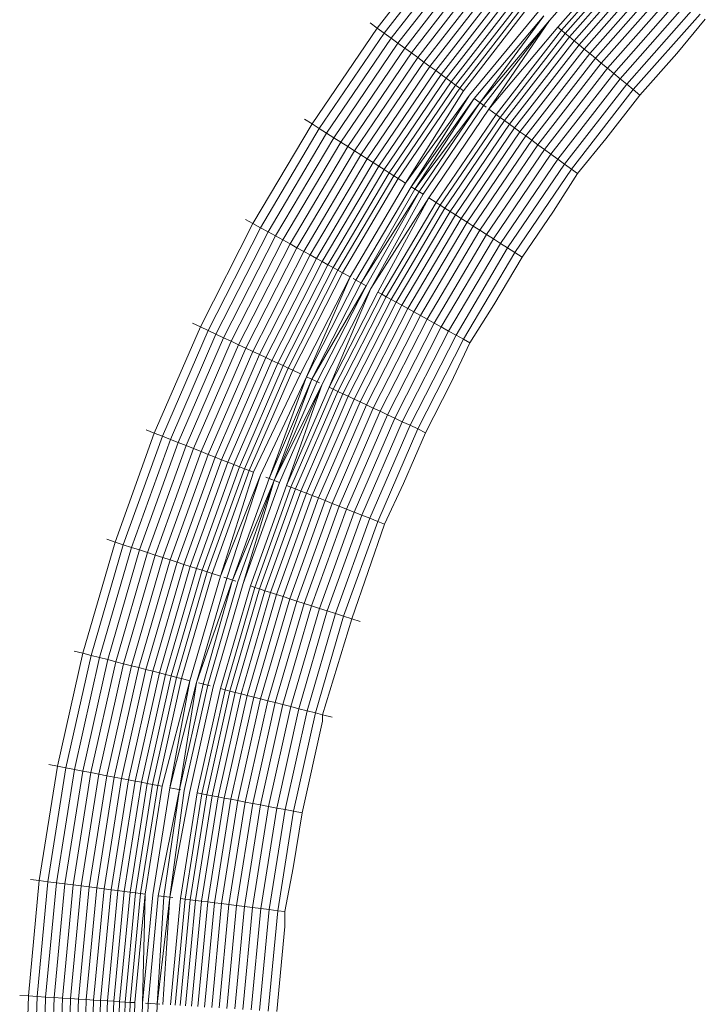
# Model space of a CAD drawing. Units: inches. Extents: x 64 to 1167, y 117 to 939.
# Tile 45 of 56: x 1129.7649 to 1129.9466, y 500.9712 to 501.2323. Entities that reach past the tile are written whole.
import ezdxf

# ---------------------------------------------------------------- set-up
doc = ezdxf.new("R2010")
doc.units = ezdxf.units.IN
doc.header["$MEASUREMENT"] = 0
doc.layers.add('A-FLOR-FIXT', color=8, linetype='Continuous', lineweight=18)

msp = doc.modelspace()

# ---------------------------------------------------------------- linework, layer by layer
at = {"layer": 'A-FLOR-FIXT'}
for p, q in [((1129.87845, 501.25434), (1129.85963, 501.23007)), ((1129.88022, 501.25287), (1129.86149, 501.22872)), ((1129.88198, 501.25142), (1129.86333, 501.22738)), ((1129.92417, 501.25352), (1129.90531, 501.23212)), ((1129.92626, 501.25156), (1129.90751, 501.2303)), ((1129.88371, 501.24999), (1129.86515, 501.22606)), ((1129.88542, 501.24858), (1129.86694, 501.22476)), ((1129.92714, 501.25073), (1129.90845, 501.22952)), ((1129.92812, 501.24981), (1129.90949, 501.22867)), ((1129.92919, 501.2488), (1129.91062, 501.22773)), ((1129.88708, 501.2472), (1129.86869, 501.22349)), ((1129.8887, 501.24586), (1129.87039, 501.22225)), ((1129.93034, 501.24772), (1129.91183, 501.22673)), ((1129.93157, 501.24657), (1129.91313, 501.22565)), ((1129.89027, 501.24456), (1129.87204, 501.22106)), ((1129.89178, 501.24331), (1129.87362, 501.2199)), ((1129.93287, 501.24535), (1129.91451, 501.22451)), ((1129.93424, 501.24406), (1129.91595, 501.22332)), ((1129.89323, 501.24212), (1129.87514, 501.2188)), ((1129.8946, 501.24098), (1129.87659, 501.21775)), ((1129.93567, 501.24272), (1129.91746, 501.22207)), ((1129.93716, 501.24132), (1129.91903, 501.22077)), ((1129.8959, 501.2399), (1129.87795, 501.21676)), ((1129.89712, 501.2389), (1129.87923, 501.21583)), ((1129.93869, 501.23988), (1129.92065, 501.21943)), ((1129.94027, 501.2384), (1129.92232, 501.21805)), ((1129.89825, 501.23796), (1129.88041, 501.21497)), ((1129.89928, 501.23711), (1129.8815, 501.21418)), ((1129.90022, 501.23633), (1129.88249, 501.21346)), ((1129.94188, 501.23689), (1129.92402, 501.21664)), ((1129.90242, 501.23451), (1129.88414, 501.21226)), ((1129.90381, 501.23336), (1129.88534, 501.21139)), ((1129.90381, 501.23336), (1129.88686, 501.21029)), ((1129.94352, 501.23535), (1129.92576, 501.21521)), ((1129.94518, 501.23379), (1129.92751, 501.21375)), ((1129.85963, 501.23007), (1129.85776, 501.23143)), ((1129.90531, 501.23212), (1129.88686, 501.21029)), ((1129.90531, 501.23212), (1129.88783, 501.20958)), ((1129.90531, 501.23212), (1129.88926, 501.20854)), ((1129.90751, 501.2303), (1129.88926, 501.20854)), ((1129.90845, 501.22952), (1129.90751, 501.2303)), ((1129.94658, 501.23247), (1129.93901, 501.22333)), ((1129.85963, 501.23007), (1129.84237, 501.20467)), ((1129.86149, 501.22872), (1129.84431, 501.20344)), ((1129.86149, 501.22872), (1129.85963, 501.23007)), ((1129.86333, 501.22738), (1129.86149, 501.22872)), ((1129.90845, 501.22952), (1129.89113, 501.20719)), ((1129.90949, 501.22867), (1129.89221, 501.2064)), ((1129.91062, 501.22773), (1129.8934, 501.20554)), ((1129.90949, 501.22867), (1129.90845, 501.22952)), ((1129.91062, 501.22773), (1129.90949, 501.22867)), ((1129.91183, 501.22673), (1129.91062, 501.22773)), ((1129.86333, 501.22738), (1129.84623, 501.20222)), ((1129.86515, 501.22606), (1129.84813, 501.20101)), ((1129.86515, 501.22606), (1129.86333, 501.22738)), ((1129.86694, 501.22476), (1129.86515, 501.22606)), ((1129.91183, 501.22673), (1129.89468, 501.20461)), ((1129.91313, 501.22565), (1129.89604, 501.20362)), ((1129.91313, 501.22565), (1129.91183, 501.22673)), ((1129.91451, 501.22451), (1129.91313, 501.22565)), ((1129.86694, 501.22476), (1129.85, 501.19983)), ((1129.86869, 501.22349), (1129.85182, 501.19867)), ((1129.86869, 501.22349), (1129.86694, 501.22476)), ((1129.87039, 501.22225), (1129.86869, 501.22349)), ((1129.91451, 501.22451), (1129.89748, 501.20257)), ((1129.91595, 501.22332), (1129.899, 501.20146)), ((1129.91595, 501.22332), (1129.91451, 501.22451)), ((1129.91746, 501.22207), (1129.91595, 501.22332)), ((1129.93901, 501.22333), (1129.92928, 501.21229)), ((1129.87039, 501.22225), (1129.8536, 501.19754)), ((1129.87204, 501.22106), (1129.85532, 501.19645)), ((1129.87362, 501.2199), (1129.85697, 501.1954)), ((1129.87204, 501.22106), (1129.87039, 501.22225)), ((1129.87362, 501.2199), (1129.87204, 501.22106)), ((1129.87514, 501.2188), (1129.87362, 501.2199)), ((1129.91746, 501.22207), (1129.90059, 501.20031)), ((1129.91903, 501.22077), (1129.90224, 501.19911)), ((1129.91903, 501.22077), (1129.91746, 501.22207)), ((1129.92065, 501.21943), (1129.91903, 501.22077)), ((1129.87514, 501.2188), (1129.85856, 501.19439)), ((1129.87659, 501.21775), (1129.86006, 501.19344)), ((1129.87659, 501.21775), (1129.87514, 501.2188)), ((1129.87795, 501.21676), (1129.87659, 501.21775)), ((1129.92065, 501.21943), (1129.90394, 501.19788)), ((1129.92232, 501.21805), (1129.90569, 501.19661)), ((1129.92232, 501.21805), (1129.92065, 501.21943)), ((1129.92402, 501.21664), (1129.92232, 501.21805)), ((1129.87795, 501.21676), (1129.86149, 501.19253)), ((1129.87923, 501.21583), (1129.86282, 501.19169)), ((1129.88041, 501.21497), (1129.86406, 501.1909)), ((1129.87923, 501.21583), (1129.87795, 501.21676)), ((1129.88041, 501.21497), (1129.87923, 501.21583)), ((1129.8815, 501.21418), (1129.88041, 501.21497)), ((1129.92402, 501.21664), (1129.90748, 501.19531)), ((1129.92576, 501.21521), (1129.9093, 501.19399)), ((1129.92576, 501.21521), (1129.92402, 501.21664)), ((1129.92751, 501.21375), (1129.92576, 501.21521)), ((1129.8815, 501.21418), (1129.86519, 501.19018)), ((1129.88249, 501.21346), (1129.86714, 501.18895)), ((1129.88414, 501.21226), (1129.86714, 501.18895)), ((1129.88414, 501.21226), (1129.86863, 501.188)), ((1129.88249, 501.21346), (1129.8815, 501.21418)), ((1129.92751, 501.21375), (1129.91114, 501.19265)), ((1129.92928, 501.21229), (1129.92026, 501.20066)), ((1129.92928, 501.21229), (1129.92751, 501.21375)), ((1129.88534, 501.21139), (1129.86863, 501.188)), ((1129.88534, 501.21139), (1129.86964, 501.18736)), ((1129.88686, 501.21029), (1129.86964, 501.18736)), ((1129.88686, 501.21029), (1129.87079, 501.18663)), ((1129.88783, 501.20958), (1129.8718, 501.18599)), ((1129.88534, 501.21139), (1129.88849, 501.2091)), ((1129.88926, 501.20854), (1129.87329, 501.18505)), ((1129.89113, 501.20719), (1129.87524, 501.18381)), ((1129.88926, 501.20854), (1129.89113, 501.20719)), ((1129.89113, 501.20719), (1129.89221, 501.2064)), ((1129.84237, 501.20467), (1129.82673, 501.17823)), ((1129.84237, 501.20467), (1129.84042, 501.20591)), ((1129.84431, 501.20344), (1129.84237, 501.20467)), ((1129.89221, 501.2064), (1129.87637, 501.18309)), ((1129.8934, 501.20554), (1129.87761, 501.1823)), ((1129.89468, 501.20461), (1129.87894, 501.18146)), ((1129.8934, 501.20554), (1129.89221, 501.2064)), ((1129.89468, 501.20461), (1129.8934, 501.20554)), ((1129.89604, 501.20362), (1129.89468, 501.20461)), ((1129.84431, 501.20344), (1129.82875, 501.17713)), ((1129.84623, 501.20222), (1129.83074, 501.17603)), ((1129.84623, 501.20222), (1129.84431, 501.20344)), ((1129.84813, 501.20101), (1129.84623, 501.20222)), ((1129.89604, 501.20362), (1129.88037, 501.18055)), ((1129.89748, 501.20257), (1129.88187, 501.1796)), ((1129.899, 501.20146), (1129.88346, 501.17859)), ((1129.89748, 501.20257), (1129.89604, 501.20362)), ((1129.899, 501.20146), (1129.89748, 501.20257)), ((1129.90059, 501.20031), (1129.899, 501.20146)), ((1129.84813, 501.20101), (1129.83271, 501.17494)), ((1129.85, 501.19983), (1129.83465, 501.17388)), ((1129.85, 501.19983), (1129.84813, 501.20101)), ((1129.85182, 501.19867), (1129.85, 501.19983)), ((1129.90059, 501.20031), (1129.88511, 501.17754)), ((1129.90224, 501.19911), (1129.88683, 501.17645)), ((1129.90224, 501.19911), (1129.90059, 501.20031)), ((1129.90394, 501.19788), (1129.90224, 501.19911)), ((1129.92026, 501.20066), (1129.9127, 501.19152)), ((1129.85182, 501.19867), (1129.83654, 501.17284)), ((1129.8536, 501.19754), (1129.83839, 501.17183)), ((1129.85532, 501.19645), (1129.84017, 501.17084)), ((1129.8536, 501.19754), (1129.85182, 501.19867)), ((1129.85532, 501.19645), (1129.8536, 501.19754)), ((1129.85697, 501.1954), (1129.85532, 501.19645)), ((1129.90394, 501.19788), (1129.88861, 501.17532)), ((1129.90569, 501.19661), (1129.89043, 501.17416)), ((1129.90569, 501.19661), (1129.90394, 501.19788)), ((1129.90748, 501.19531), (1129.90569, 501.19661)), ((1129.85697, 501.1954), (1129.84189, 501.1699)), ((1129.85856, 501.19439), (1129.84354, 501.16899)), ((1129.85856, 501.19439), (1129.85697, 501.1954)), ((1129.86006, 501.19344), (1129.85856, 501.19439)), ((1129.90748, 501.19531), (1129.8923, 501.17298)), ((1129.9093, 501.19399), (1129.8942, 501.17177)), ((1129.9093, 501.19399), (1129.90748, 501.19531)), ((1129.91114, 501.19265), (1129.9093, 501.19399)), ((1129.86006, 501.19344), (1129.8451, 501.16813)), ((1129.86149, 501.19253), (1129.84658, 501.16732)), ((1129.86282, 501.19169), (1129.84796, 501.16656)), ((1129.86149, 501.19253), (1129.86006, 501.19344)), ((1129.86282, 501.19169), (1129.86149, 501.19253)), ((1129.86406, 501.1909), (1129.86282, 501.19169)), ((1129.91114, 501.19265), (1129.89612, 501.17055)), ((1129.9127, 501.19152), (1129.90634, 501.18149)), ((1129.9127, 501.19152), (1129.91114, 501.19265)), ((1129.86406, 501.1909), (1129.84924, 501.16586)), ((1129.86519, 501.19018), (1129.85042, 501.16521)), ((1129.86714, 501.18895), (1129.85245, 501.1641)), ((1129.86519, 501.19018), (1129.86406, 501.1909)), ((1129.86714, 501.18895), (1129.86519, 501.19018)), ((1129.86863, 501.188), (1129.85399, 501.16325)), ((1129.86964, 501.18736), (1129.85537, 501.16249)), ((1129.87079, 501.18663), (1129.85537, 501.16249)), ((1129.87079, 501.18663), (1129.85669, 501.16176)), ((1129.8718, 501.18599), (1129.85799, 501.16105)), ((1129.86863, 501.188), (1129.8718, 501.18599)), ((1129.87329, 501.18505), (1129.85799, 501.16105)), ((1129.87329, 501.18505), (1129.85978, 501.16007)), ((1129.87524, 501.18381), (1129.86085, 501.15948)), ((1129.87524, 501.18381), (1129.87329, 501.18505)), ((1129.87637, 501.18309), (1129.87524, 501.18381)), ((1129.87637, 501.18309), (1129.86203, 501.15883)), ((1129.87761, 501.1823), (1129.86331, 501.15812)), ((1129.87894, 501.18146), (1129.86469, 501.15736)), ((1129.87761, 501.1823), (1129.87637, 501.18309)), ((1129.87894, 501.18146), (1129.87761, 501.1823)), ((1129.88037, 501.18055), (1129.87894, 501.18146)), ((1129.90634, 501.18149), (1129.89806, 501.16932)), ((1129.82673, 501.17823), (1129.81279, 501.15087)), ((1129.82673, 501.17823), (1129.82471, 501.17935)), ((1129.82875, 501.17713), (1129.82673, 501.17823)), ((1129.88037, 501.18055), (1129.86617, 501.15655)), ((1129.88187, 501.1796), (1129.86774, 501.15569)), ((1129.88346, 501.17859), (1129.86938, 501.15479)), ((1129.88187, 501.1796), (1129.88037, 501.18055)), ((1129.88346, 501.17859), (1129.88187, 501.1796)), ((1129.88511, 501.17754), (1129.88346, 501.17859)), ((1129.82875, 501.17713), (1129.81487, 501.14989)), ((1129.83074, 501.17603), (1129.81693, 501.14892)), ((1129.83074, 501.17603), (1129.82875, 501.17713)), ((1129.83271, 501.17494), (1129.83074, 501.17603)), ((1129.88511, 501.17754), (1129.8711, 501.15384)), ((1129.88683, 501.17645), (1129.87288, 501.15286)), ((1129.88683, 501.17645), (1129.88511, 501.17754)), ((1129.88861, 501.17532), (1129.88683, 501.17645)), ((1129.83271, 501.17494), (1129.81896, 501.14796)), ((1129.83465, 501.17388), (1129.82096, 501.14702)), ((1129.83654, 501.17284), (1129.82292, 501.1461)), ((1129.83465, 501.17388), (1129.83271, 501.17494)), ((1129.83654, 501.17284), (1129.83465, 501.17388)), ((1129.83839, 501.17183), (1129.83654, 501.17284)), ((1129.88861, 501.17532), (1129.87473, 501.15185)), ((1129.89043, 501.17416), (1129.87662, 501.15081)), ((1129.8923, 501.17298), (1129.87856, 501.14974)), ((1129.89043, 501.17416), (1129.88861, 501.17532)), ((1129.8923, 501.17298), (1129.89043, 501.17416)), ((1129.8942, 501.17177), (1129.8923, 501.17298)), ((1129.83839, 501.17183), (1129.82482, 501.1452)), ((1129.84017, 501.17084), (1129.82667, 501.14434)), ((1129.84017, 501.17084), (1129.83839, 501.17183)), ((1129.84189, 501.1699), (1129.84017, 501.17084)), ((1129.8942, 501.17177), (1129.88053, 501.14866)), ((1129.89612, 501.17055), (1129.88253, 501.14756)), ((1129.89612, 501.17055), (1129.8942, 501.17177)), ((1129.89806, 501.16932), (1129.89612, 501.17055)), ((1129.84189, 501.1699), (1129.82844, 501.1435)), ((1129.84354, 501.16899), (1129.83014, 501.1427)), ((1129.8451, 501.16813), (1129.83175, 501.14194)), ((1129.84354, 501.16899), (1129.84189, 501.1699)), ((1129.8451, 501.16813), (1129.84354, 501.16899)), ((1129.84658, 501.16732), (1129.8451, 501.16813)), ((1129.89806, 501.16932), (1129.89057, 501.15666)), ((1129.84658, 501.16732), (1129.83328, 501.14123)), ((1129.84796, 501.16656), (1129.83471, 501.14055)), ((1129.84924, 501.16586), (1129.83603, 501.13993)), ((1129.85042, 501.16521), (1129.83725, 501.13936)), ((1129.84796, 501.16656), (1129.84658, 501.16732)), ((1129.84924, 501.16586), (1129.84796, 501.16656)), ((1129.85042, 501.16521), (1129.84924, 501.16586)), ((1129.85245, 501.1641), (1129.85042, 501.16521)), ((1129.85245, 501.1641), (1129.83934, 501.13837)), ((1129.85245, 501.1641), (1129.84094, 501.13762)), ((1129.85399, 501.16325), (1129.84094, 501.13762)), ((1129.85537, 501.16249), (1129.84236, 501.13695)), ((1129.85328, 501.16364), (1129.85669, 501.16176)), ((1129.85669, 501.16176), (1129.84236, 501.13695)), ((1129.85669, 501.16176), (1129.84372, 501.13631)), ((1129.85799, 501.16105), (1129.84506, 501.13568)), ((1129.85799, 501.16105), (1129.84691, 501.13481)), ((1129.85978, 501.16007), (1129.84691, 501.13481)), ((1129.86085, 501.15948), (1129.85978, 501.16007)), ((1129.86085, 501.15948), (1129.84801, 501.13429)), ((1129.86203, 501.15883), (1129.84923, 501.13372)), ((1129.86331, 501.15812), (1129.85056, 501.13309)), ((1129.86469, 501.15736), (1129.85199, 501.13242)), ((1129.86203, 501.15883), (1129.86085, 501.15948)), ((1129.86331, 501.15812), (1129.86203, 501.15883)), ((1129.86469, 501.15736), (1129.86331, 501.15812)), ((1129.86617, 501.15655), (1129.86469, 501.15736)), ((1129.86617, 501.15655), (1129.85351, 501.1317)), ((1129.86774, 501.15569), (1129.85513, 501.13094)), ((1129.86938, 501.15479), (1129.85683, 501.13015)), ((1129.86774, 501.15569), (1129.86617, 501.15655)), ((1129.86938, 501.15479), (1129.86774, 501.15569)), ((1129.8711, 501.15384), (1129.86938, 501.15479)), ((1129.89057, 501.15666), (1129.88421, 501.14663)), ((1129.81279, 501.15087), (1129.8107, 501.15185)), ((1129.8711, 501.15384), (1129.8586, 501.12931)), ((1129.87288, 501.15286), (1129.86044, 501.12844)), ((1129.87473, 501.15185), (1129.86235, 501.12755)), ((1129.87288, 501.15286), (1129.8711, 501.15384)), ((1129.87473, 501.15185), (1129.87288, 501.15286)), ((1129.87662, 501.15081), (1129.87473, 501.15185)), ((1129.81279, 501.15087), (1129.80059, 501.12268)), ((1129.81487, 501.14989), (1129.80273, 501.12183)), ((1129.81487, 501.14989), (1129.81279, 501.15087)), ((1129.81693, 501.14892), (1129.81487, 501.14989)), ((1129.87662, 501.15081), (1129.8643, 501.12663)), ((1129.87856, 501.14974), (1129.8663, 501.12569)), ((1129.87856, 501.14974), (1129.87662, 501.15081)), ((1129.88053, 501.14866), (1129.87856, 501.14974)), ((1129.81693, 501.14892), (1129.80485, 501.121)), ((1129.81896, 501.14796), (1129.80694, 501.12017)), ((1129.82096, 501.14702), (1129.80899, 501.11935)), ((1129.81896, 501.14796), (1129.81693, 501.14892)), ((1129.82096, 501.14702), (1129.81896, 501.14796)), ((1129.82292, 501.1461), (1129.82096, 501.14702)), ((1129.88053, 501.14866), (1129.86834, 501.12473)), ((1129.88253, 501.14756), (1129.8704, 501.12376)), ((1129.88421, 501.14663), (1129.87916, 501.13589)), ((1129.88253, 501.14756), (1129.88053, 501.14866)), ((1129.88421, 501.14663), (1129.88253, 501.14756)), ((1129.82292, 501.1461), (1129.811, 501.11856)), ((1129.82482, 501.1452), (1129.81296, 501.11778)), ((1129.82667, 501.14434), (1129.81485, 501.11703)), ((1129.82482, 501.1452), (1129.82292, 501.1461)), ((1129.82667, 501.14434), (1129.82482, 501.1452)), ((1129.82844, 501.1435), (1129.82667, 501.14434)), ((1129.82844, 501.1435), (1129.81667, 501.11631)), ((1129.83014, 501.1427), (1129.81842, 501.11562)), ((1129.83175, 501.14194), (1129.82008, 501.11496)), ((1129.83014, 501.1427), (1129.82844, 501.1435)), ((1129.83175, 501.14194), (1129.83014, 501.1427)), ((1129.83328, 501.14123), (1129.83175, 501.14194)), ((1129.83328, 501.14123), (1129.82165, 501.11434)), ((1129.83471, 501.14055), (1129.82312, 501.11376)), ((1129.83603, 501.13993), (1129.82448, 501.11322)), ((1129.83725, 501.13936), (1129.82573, 501.11273)), ((1129.83471, 501.14055), (1129.83328, 501.14123)), ((1129.83603, 501.13993), (1129.83471, 501.14055)), ((1129.83725, 501.13936), (1129.83603, 501.13993)), ((1129.83934, 501.13837), (1129.83725, 501.13936)), ((1129.83934, 501.13837), (1129.82686, 501.11228)), ((1129.84094, 501.13762), (1129.82876, 501.11153)), ((1129.84094, 501.13762), (1129.83098, 501.11065)), ((1129.84236, 501.13695), (1129.83098, 501.11065)), ((1129.84236, 501.13695), (1129.83238, 501.1101)), ((1129.84372, 501.13631), (1129.83238, 501.1101)), ((1129.84094, 501.13762), (1129.84433, 501.13603)), ((1129.84506, 501.13568), (1129.83238, 501.1101)), ((1129.84506, 501.13568), (1129.83376, 501.10955)), ((1129.84506, 501.13568), (1129.83565, 501.1088)), ((1129.84691, 501.13481), (1129.83565, 501.1088)), ((1129.84801, 501.13429), (1129.83679, 501.10835)), ((1129.84923, 501.13372), (1129.83804, 501.10785)), ((1129.84691, 501.13481), (1129.84801, 501.13429)), ((1129.84801, 501.13429), (1129.84923, 501.13372)), ((1129.84923, 501.13372), (1129.85056, 501.13309)), ((1129.87916, 501.13589), (1129.87248, 501.12278)), ((1129.85056, 501.13309), (1129.8394, 501.10731)), ((1129.85199, 501.13242), (1129.84087, 501.10673)), ((1129.85351, 501.1317), (1129.84244, 501.10611)), ((1129.85056, 501.13309), (1129.85199, 501.13242)), ((1129.85351, 501.1317), (1129.85199, 501.13242)), ((1129.85513, 501.13094), (1129.85351, 501.1317)), ((1129.85513, 501.13094), (1129.8441, 501.10546)), ((1129.85683, 501.13015), (1129.84584, 501.10476)), ((1129.8586, 501.12931), (1129.84767, 501.10404)), ((1129.86044, 501.12844), (1129.84956, 501.10329)), ((1129.85683, 501.13015), (1129.85513, 501.13094)), ((1129.8586, 501.12931), (1129.85683, 501.13015)), ((1129.86044, 501.12844), (1129.8586, 501.12931)), ((1129.86235, 501.12755), (1129.86044, 501.12844)), ((1129.86235, 501.12755), (1129.85151, 501.10252)), ((1129.8643, 501.12663), (1129.85352, 501.10172)), ((1129.8643, 501.12663), (1129.86235, 501.12755)), ((1129.8663, 501.12569), (1129.8643, 501.12663)), ((1129.80059, 501.12268), (1129.79844, 501.12353)), ((1129.8663, 501.12569), (1129.85558, 501.10091)), ((1129.86834, 501.12473), (1129.85767, 501.10008)), ((1129.8704, 501.12376), (1129.85979, 501.09924)), ((1129.86834, 501.12473), (1129.8663, 501.12569)), ((1129.8704, 501.12376), (1129.86834, 501.12473)), ((1129.87248, 501.12278), (1129.8704, 501.12376)), ((1129.80059, 501.12268), (1129.79019, 501.09378)), ((1129.80273, 501.12183), (1129.79237, 501.09307)), ((1129.80485, 501.121), (1129.79454, 501.09237)), ((1129.80273, 501.12183), (1129.80059, 501.12268)), ((1129.80485, 501.121), (1129.80273, 501.12183)), ((1129.80694, 501.12017), (1129.80485, 501.121)), ((1129.87248, 501.12278), (1129.86663, 501.10928)), ((1129.80694, 501.12017), (1129.79668, 501.09167)), ((1129.80899, 501.11935), (1129.79878, 501.09099)), ((1129.811, 501.11856), (1129.80084, 501.09032)), ((1129.80899, 501.11935), (1129.80694, 501.12017)), ((1129.811, 501.11856), (1129.80899, 501.11935)), ((1129.81296, 501.11778), (1129.811, 501.11856)), ((1129.81296, 501.11778), (1129.80284, 501.08967)), ((1129.81485, 501.11703), (1129.80477, 501.08904)), ((1129.81667, 501.11631), (1129.80664, 501.08844)), ((1129.81842, 501.11562), (1129.80842, 501.08786)), ((1129.81485, 501.11703), (1129.81296, 501.11778)), ((1129.81667, 501.11631), (1129.81485, 501.11703)), ((1129.81842, 501.11562), (1129.81667, 501.11631)), ((1129.82008, 501.11496), (1129.81842, 501.11562)), ((1129.82008, 501.11496), (1129.81012, 501.08731)), ((1129.82165, 501.11434), (1129.81173, 501.08679)), ((1129.82312, 501.11376), (1129.81323, 501.0863)), ((1129.82448, 501.11322), (1129.81462, 501.08584)), ((1129.82573, 501.11273), (1129.8159, 501.08543)), ((1129.82165, 501.11434), (1129.82008, 501.11496)), ((1129.82312, 501.11376), (1129.82165, 501.11434)), ((1129.82448, 501.11322), (1129.82312, 501.11376)), ((1129.82573, 501.11273), (1129.82448, 501.11322)), ((1129.82686, 501.11228), (1129.82573, 501.11273)), ((1129.82686, 501.11228), (1129.8181, 501.08472)), ((1129.82876, 501.11153), (1129.8181, 501.08472)), ((1129.82876, 501.11153), (1129.81978, 501.08417)), ((1129.83098, 501.11065), (1129.82127, 501.08368)), ((1129.83238, 501.1101), (1129.82127, 501.08368)), ((1129.83238, 501.1101), (1129.8227, 501.08322)), ((1129.83238, 501.1101), (1129.82411, 501.08276)), ((1129.83014, 501.11098), (1129.83376, 501.10955)), ((1129.83376, 501.10955), (1129.82411, 501.08276)), ((1129.83565, 501.1088), (1129.82605, 501.08213)), ((1129.83679, 501.10835), (1129.82721, 501.08175)), ((1129.83804, 501.10785), (1129.82849, 501.08134)), ((1129.83679, 501.10835), (1129.83565, 501.1088)), ((1129.83804, 501.10785), (1129.83679, 501.10835)), ((1129.8394, 501.10731), (1129.83804, 501.10785)), ((1129.86663, 501.10928), (1129.86158, 501.09853)), ((1129.8394, 501.10731), (1129.82989, 501.08088)), ((1129.84087, 501.10673), (1129.83139, 501.0804)), ((1129.84244, 501.10611), (1129.83299, 501.07988)), ((1129.8441, 501.10546), (1129.83469, 501.07932)), ((1129.84087, 501.10673), (1129.8394, 501.10731)), ((1129.84244, 501.10611), (1129.84087, 501.10673)), ((1129.84244, 501.10611), (1129.8441, 501.10546)), ((1129.8441, 501.10546), (1129.84584, 501.10476)), ((1129.84584, 501.10476), (1129.83647, 501.07874)), ((1129.84767, 501.10404), (1129.83834, 501.07814)), ((1129.84956, 501.10329), (1129.84028, 501.07751)), ((1129.85151, 501.10252), (1129.84228, 501.07686)), ((1129.84584, 501.10476), (1129.84767, 501.10404)), ((1129.84767, 501.10404), (1129.84956, 501.10329)), ((1129.84956, 501.10329), (1129.85151, 501.10252)), ((1129.85151, 501.10252), (1129.85352, 501.10172)), ((1129.85352, 501.10172), (1129.84433, 501.07619)), ((1129.85558, 501.10091), (1129.84643, 501.07551)), ((1129.85767, 501.10008), (1129.84857, 501.07481)), ((1129.85352, 501.10172), (1129.85558, 501.10091)), ((1129.85558, 501.10091), (1129.85767, 501.10008)), ((1129.85767, 501.10008), (1129.85979, 501.09924)), ((1129.85979, 501.09924), (1129.85074, 501.07411)), ((1129.86158, 501.09853), (1129.85293, 501.0734)), ((1129.85979, 501.09924), (1129.86158, 501.09853)), ((1129.79019, 501.09378), (1129.78799, 501.0945)), ((1129.79019, 501.09378), (1129.78162, 501.06429)), ((1129.79237, 501.09307), (1129.78384, 501.06372)), ((1129.79454, 501.09237), (1129.78605, 501.06315)), ((1129.79237, 501.09307), (1129.79019, 501.09378)), ((1129.79454, 501.09237), (1129.79237, 501.09307)), ((1129.79668, 501.09167), (1129.79454, 501.09237)), ((1129.79668, 501.09167), (1129.78823, 501.06259)), ((1129.79878, 501.09099), (1129.79037, 501.06204)), ((1129.80084, 501.09032), (1129.79246, 501.06151)), ((1129.80284, 501.08967), (1129.7945, 501.06098)), ((1129.79878, 501.09099), (1129.79668, 501.09167)), ((1129.80084, 501.09032), (1129.79878, 501.09099)), ((1129.80284, 501.08967), (1129.80084, 501.09032)), ((1129.80477, 501.08904), (1129.80284, 501.08967)), ((1129.80477, 501.08904), (1129.79647, 501.06048)), ((1129.80664, 501.08844), (1129.79837, 501.05999)), ((1129.80842, 501.08786), (1129.80019, 501.05952)), ((1129.81012, 501.08731), (1129.80192, 501.05908)), ((1129.81173, 501.08679), (1129.80355, 501.05866)), ((1129.80664, 501.08844), (1129.80477, 501.08904)), ((1129.80842, 501.08786), (1129.80664, 501.08844)), ((1129.81012, 501.08731), (1129.80842, 501.08786)), ((1129.81173, 501.08679), (1129.81012, 501.08731)), ((1129.81323, 501.0863), (1129.81173, 501.08679)), ((1129.81323, 501.0863), (1129.80508, 501.05827)), ((1129.81462, 501.08584), (1129.8065, 501.0579)), ((1129.8159, 501.08543), (1129.80781, 501.05757)), ((1129.8181, 501.08472), (1129.81004, 501.05699)), ((1129.81978, 501.08417), (1129.81175, 501.05655)), ((1129.81462, 501.08584), (1129.81323, 501.0863)), ((1129.8159, 501.08543), (1129.81462, 501.08584)), ((1129.8181, 501.08472), (1129.8159, 501.08543)), ((1129.819, 501.08442), (1129.8222, 501.08338)), ((1129.82127, 501.08368), (1129.81175, 501.05655)), ((1129.82127, 501.08368), (1129.81349, 501.05611)), ((1129.8227, 501.08322), (1129.81473, 501.05579)), ((1129.82411, 501.08276), (1129.81617, 501.05542)), ((1129.82605, 501.08213), (1129.81815, 501.05491)), ((1129.82721, 501.08175), (1129.81933, 501.05461)), ((1129.82721, 501.08175), (1129.82605, 501.08213)), ((1129.82849, 501.08134), (1129.82721, 501.08175)), ((1129.82849, 501.08134), (1129.82063, 501.05427)), ((1129.82989, 501.08088), (1129.82205, 501.05391)), ((1129.83139, 501.0804), (1129.82358, 501.05352)), ((1129.83299, 501.07988), (1129.82521, 501.0531)), ((1129.83469, 501.07932), (1129.82694, 501.05265)), ((1129.82989, 501.08088), (1129.82849, 501.08134)), ((1129.83647, 501.07874), (1129.82876, 501.05219)), ((1129.83139, 501.0804), (1129.82989, 501.08088)), ((1129.83299, 501.07988), (1129.83139, 501.0804)), ((1129.83469, 501.07932), (1129.83299, 501.07988)), ((1129.83647, 501.07874), (1129.83469, 501.07932)), ((1129.83834, 501.07814), (1129.83647, 501.07874)), ((1129.83834, 501.07814), (1129.83066, 501.0517)), ((1129.84028, 501.07751), (1129.83263, 501.05119)), ((1129.84228, 501.07686), (1129.83467, 501.05067)), ((1129.84433, 501.07619), (1129.83676, 501.05013)), ((1129.84028, 501.07751), (1129.83834, 501.07814)), ((1129.84228, 501.07686), (1129.84028, 501.07751)), ((1129.84433, 501.07619), (1129.84228, 501.07686)), ((1129.84643, 501.07551), (1129.84433, 501.07619)), ((1129.84643, 501.07551), (1129.8389, 501.04958)), ((1129.84857, 501.07481), (1129.84108, 501.04902)), ((1129.85074, 501.07411), (1129.84329, 501.04846)), ((1129.84857, 501.07481), (1129.84643, 501.07551)), ((1129.85074, 501.07411), (1129.84857, 501.07481)), ((1129.85293, 501.0734), (1129.85074, 501.07411)), ((1129.85293, 501.0734), (1129.84515, 501.04798)), ((1129.85512, 501.07269), (1129.85293, 501.0734)), ((1129.78162, 501.06429), (1129.77492, 501.03432)), ((1129.78384, 501.06372), (1129.77718, 501.03389)), ((1129.78162, 501.06429), (1129.77938, 501.06486)), ((1129.78605, 501.06315), (1129.77941, 501.03346)), ((1129.78384, 501.06372), (1129.78162, 501.06429)), ((1129.78605, 501.06315), (1129.78384, 501.06372)), ((1129.78823, 501.06259), (1129.78605, 501.06315)), ((1129.78823, 501.06259), (1129.78162, 501.03304)), ((1129.79037, 501.06204), (1129.78379, 501.03262)), ((1129.79246, 501.06151), (1129.78592, 501.03222)), ((1129.7945, 501.06098), (1129.78798, 501.03182)), ((1129.79037, 501.06204), (1129.78823, 501.06259)), ((1129.79647, 501.06048), (1129.78998, 501.03144)), ((1129.79246, 501.06151), (1129.79037, 501.06204)), ((1129.79246, 501.06151), (1129.7945, 501.06098)), ((1129.7945, 501.06098), (1129.79647, 501.06048)), ((1129.79647, 501.06048), (1129.79837, 501.05999)), ((1129.79837, 501.05999), (1129.79191, 501.03108)), ((1129.80019, 501.05952), (1129.79376, 501.03072)), ((1129.80192, 501.05908), (1129.79551, 501.03039)), ((1129.80355, 501.05866), (1129.79716, 501.03007)), ((1129.79837, 501.05999), (1129.80019, 501.05952)), ((1129.80508, 501.05827), (1129.79872, 501.02978)), ((1129.8065, 501.0579), (1129.80015, 501.0295)), ((1129.80019, 501.05952), (1129.80192, 501.05908)), ((1129.80192, 501.05908), (1129.80355, 501.05866)), ((1129.80355, 501.05866), (1129.80508, 501.05827)), ((1129.80508, 501.05827), (1129.8065, 501.0579)), ((1129.8065, 501.0579), (1129.80781, 501.05757)), ((1129.80781, 501.05757), (1129.80148, 501.02925)), ((1129.81004, 501.05699), (1129.80267, 501.02902)), ((1129.81004, 501.05699), (1129.80468, 501.02864)), ((1129.81175, 501.05655), (1129.80468, 501.02864)), ((1129.81175, 501.05655), (1129.80724, 501.02815)), ((1129.81349, 501.05611), (1129.80724, 501.02815)), ((1129.80781, 501.05757), (1129.81004, 501.05699)), ((1129.81473, 501.05579), (1129.8085, 501.02791)), ((1129.81617, 501.05542), (1129.80996, 501.02763)), ((1129.81228, 501.05642), (1129.81538, 501.05562)), ((1129.81815, 501.05491), (1129.81196, 501.02725)), ((1129.81933, 501.05461), (1129.81316, 501.02702)), ((1129.82063, 501.05427), (1129.81448, 501.02677)), ((1129.82205, 501.05391), (1129.81592, 501.0265)), ((1129.82358, 501.05352), (1129.81747, 501.0262)), ((1129.81933, 501.05461), (1129.81815, 501.05491)), ((1129.82521, 501.0531), (1129.81913, 501.02588)), ((1129.82063, 501.05427), (1129.81933, 501.05461)), ((1129.82205, 501.05391), (1129.82063, 501.05427)), ((1129.82694, 501.05265), (1129.82088, 501.02555)), ((1129.82358, 501.05352), (1129.82205, 501.05391)), ((1129.82521, 501.0531), (1129.82358, 501.05352)), ((1129.82694, 501.05265), (1129.82521, 501.0531)), ((1129.82876, 501.05219), (1129.82694, 501.05265)), ((1129.82876, 501.05219), (1129.82273, 501.0252)), ((1129.83066, 501.0517), (1129.82465, 501.02483)), ((1129.83263, 501.05119), (1129.82665, 501.02445)), ((1129.83467, 501.05067), (1129.82872, 501.02405)), ((1129.83066, 501.0517), (1129.82876, 501.05219)), ((1129.83263, 501.05119), (1129.83066, 501.0517)), ((1129.83676, 501.05013), (1129.83084, 501.02365)), ((1129.83467, 501.05067), (1129.83263, 501.05119)), ((1129.83676, 501.05013), (1129.83467, 501.05067)), ((1129.8389, 501.04958), (1129.83676, 501.05013)), ((1129.8389, 501.04958), (1129.83301, 501.02323)), ((1129.84108, 501.04902), (1129.83522, 501.02281)), ((1129.84329, 501.04846), (1129.83746, 501.02239)), ((1129.84108, 501.04902), (1129.8389, 501.04958)), ((1129.84329, 501.04846), (1129.84108, 501.04902)), ((1129.84515, 501.04798), (1129.84329, 501.04846)), ((1129.84775, 501.04731), (1129.84515, 501.04798)), ((1129.84515, 501.04798), (1129.84515, 501.04627)), ((1129.83972, 501.02196), (1129.84515, 501.04627)), ((1129.77492, 501.03432), (1129.77265, 501.03475)), ((1129.77492, 501.03432), (1129.77011, 501.00398)), ((1129.77718, 501.03389), (1129.77239, 501.00369)), ((1129.77941, 501.03346), (1129.77465, 501.00341)), ((1129.77718, 501.03389), (1129.77492, 501.03432)), ((1129.78162, 501.03304), (1129.77689, 501.00313)), ((1129.77941, 501.03346), (1129.77718, 501.03389)), ((1129.78379, 501.03262), (1129.77908, 501.00285)), ((1129.78162, 501.03304), (1129.77941, 501.03346)), ((1129.78592, 501.03222), (1129.78122, 501.00258)), ((1129.78379, 501.03262), (1129.78162, 501.03304)), ((1129.78798, 501.03182), (1129.78331, 501.00232)), ((1129.78592, 501.03222), (1129.78379, 501.03262)), ((1129.78798, 501.03182), (1129.78592, 501.03222)), ((1129.78998, 501.03144), (1129.78798, 501.03182)), ((1129.78998, 501.03144), (1129.78533, 501.00206)), ((1129.79191, 501.03108), (1129.78728, 501.00181)), ((1129.79376, 501.03072), (1129.78914, 501.00158)), ((1129.79191, 501.03108), (1129.78998, 501.03144)), ((1129.79551, 501.03039), (1129.79091, 501.00135)), ((1129.79376, 501.03072), (1129.79191, 501.03108)), ((1129.79716, 501.03007), (1129.79258, 501.00114)), ((1129.79551, 501.03039), (1129.79376, 501.03072)), ((1129.79872, 501.02978), (1129.79415, 501.00095)), ((1129.79716, 501.03007), (1129.79551, 501.03039)), ((1129.80015, 501.0295), (1129.7956, 501.00076)), ((1129.80148, 501.02925), (1129.79694, 501.00059)), ((1129.79872, 501.02978), (1129.79716, 501.03007)), ((1129.80015, 501.0295), (1129.79872, 501.02978)), ((1129.80148, 501.02925), (1129.80015, 501.0295)), ((1129.80267, 501.02902), (1129.80148, 501.02925)), ((1129.80267, 501.02902), (1129.79815, 501.00044)), ((1129.80468, 501.02864), (1129.80017, 501.00018)), ((1129.80724, 501.02815), (1129.80164, 501)), ((1129.80724, 501.02815), (1129.80314, 500.99981)), ((1129.80468, 501.02864), (1129.80761, 501.02808)), ((1129.8085, 501.02791), (1129.8047, 500.99961)), ((1129.80996, 501.02763), (1129.8047, 500.99961)), ((1129.81196, 501.02725), (1129.80753, 500.99926)), ((1129.81316, 501.02702), (1129.80874, 500.9991)), ((1129.81448, 501.02677), (1129.81007, 500.99893)), ((1129.81316, 501.02702), (1129.81196, 501.02725)), ((1129.81448, 501.02677), (1129.81316, 501.02702)), ((1129.81592, 501.0265), (1129.81448, 501.02677)), ((1129.81592, 501.0265), (1129.81153, 500.99875)), ((1129.81747, 501.0262), (1129.81309, 500.99855)), ((1129.81913, 501.02588), (1129.81477, 500.99834)), ((1129.81747, 501.0262), (1129.81592, 501.0265)), ((1129.82088, 501.02555), (1129.81654, 500.99812)), ((1129.81913, 501.02588), (1129.81747, 501.0262)), ((1129.82273, 501.0252), (1129.8184, 500.99788)), ((1129.82088, 501.02555), (1129.81913, 501.02588)), ((1129.82465, 501.02483), (1129.82034, 500.99764)), ((1129.82273, 501.0252), (1129.82088, 501.02555)), ((1129.82665, 501.02445), (1129.82237, 500.99738)), ((1129.82465, 501.02483), (1129.82273, 501.0252)), ((1129.82872, 501.02405), (1129.82445, 500.99712)), ((1129.82665, 501.02445), (1129.82465, 501.02483)), ((1129.82872, 501.02405), (1129.82665, 501.02445)), ((1129.83084, 501.02365), (1129.82872, 501.02405)), ((1129.83084, 501.02365), (1129.8266, 500.99685)), ((1129.83301, 501.02323), (1129.82879, 500.99657)), ((1129.83301, 501.02323), (1129.83084, 501.02365)), ((1129.83522, 501.02281), (1129.83102, 500.99629)), ((1129.83522, 501.02281), (1129.83301, 501.02323)), ((1129.83746, 501.02239), (1129.83328, 500.996)), ((1129.83746, 501.02239), (1129.83522, 501.02281)), ((1129.83972, 501.02196), (1129.83742, 501.00742)), ((1129.83972, 501.02196), (1129.83746, 501.02239)), ((1129.83742, 501.00742), (1129.83519, 500.99576)), ((1129.77011, 501.00398), (1129.76722, 500.97341)), ((1129.77011, 501.00398), (1129.76782, 501.00427)), ((1129.77239, 501.00369), (1129.76952, 500.97326)), ((1129.77239, 501.00369), (1129.77011, 501.00398)), ((1129.77465, 501.00341), (1129.77179, 500.97312)), ((1129.77465, 501.00341), (1129.77239, 501.00369)), ((1129.77689, 501.00313), (1129.77404, 500.97298)), ((1129.77689, 501.00313), (1129.77465, 501.00341)), ((1129.77908, 501.00285), (1129.77689, 501.00313)), ((1129.77908, 501.00285), (1129.77624, 500.97284)), ((1129.78122, 501.00258), (1129.7784, 500.9727)), ((1129.78122, 501.00258), (1129.77908, 501.00285)), ((1129.78331, 501.00232), (1129.7805, 500.97257)), ((1129.78331, 501.00232), (1129.78122, 501.00258)), ((1129.78533, 501.00206), (1129.78253, 500.97244)), ((1129.78533, 501.00206), (1129.78331, 501.00232)), ((1129.78728, 501.00181), (1129.78449, 500.97232)), ((1129.78728, 501.00181), (1129.78533, 501.00206)), ((1129.78914, 501.00158), (1129.78636, 500.9722)), ((1129.78914, 501.00158), (1129.78728, 501.00181)), ((1129.79091, 501.00135), (1129.78814, 500.97209)), ((1129.79091, 501.00135), (1129.78914, 501.00158)), ((1129.79258, 501.00114), (1129.78983, 500.97198)), ((1129.79258, 501.00114), (1129.79091, 501.00135)), ((1129.79415, 501.00095), (1129.7914, 500.97188)), ((1129.79415, 501.00095), (1129.79258, 501.00114)), ((1129.7956, 501.00076), (1129.79286, 500.97179)), ((1129.7956, 501.00076), (1129.79415, 501.00095)), ((1129.79694, 501.00059), (1129.79421, 500.97171)), ((1129.79815, 501.00044), (1129.79542, 500.97163)), ((1129.79694, 501.00059), (1129.7956, 501.00076)), ((1129.79815, 501.00044), (1129.79694, 501.00059)), ((1129.79815, 501.00044), (1129.79746, 500.9715)), ((1129.80017, 501.00018), (1129.79746, 500.9715)), ((1129.80164, 501), (1129.79894, 500.97141)), ((1129.80314, 500.99981), (1129.80134, 500.97126)), ((1129.8047, 500.99961), (1129.80134, 500.97126)), ((1129.80164, 501), (1129.8055, 500.99951)), ((1129.8047, 500.99961), (1129.80282, 500.97117)), ((1129.80753, 500.99926), (1129.80486, 500.97104)), ((1129.80874, 500.9991), (1129.80608, 500.97096)), ((1129.81007, 500.99893), (1129.80742, 500.97088)), ((1129.80874, 500.9991), (1129.80753, 500.99926)), ((1129.81007, 500.99893), (1129.80874, 500.9991)), ((1129.81153, 500.99875), (1129.80888, 500.97078)), ((1129.81153, 500.99875), (1129.81007, 500.99893)), ((1129.81309, 500.99855), (1129.81046, 500.97069)), ((1129.81309, 500.99855), (1129.81153, 500.99875)), ((1129.81477, 500.99834), (1129.81214, 500.97058)), ((1129.81477, 500.99834), (1129.81309, 500.99855)), ((1129.81654, 500.99812), (1129.81392, 500.97047)), ((1129.81654, 500.99812), (1129.81477, 500.99834)), ((1129.8184, 500.99788), (1129.8158, 500.97035)), ((1129.8184, 500.99788), (1129.81654, 500.99812)), ((1129.82034, 500.99764), (1129.8184, 500.99788)), ((1129.82034, 500.99764), (1129.81775, 500.97023)), ((1129.82237, 500.99738), (1129.81979, 500.9701)), ((1129.82237, 500.99738), (1129.82034, 500.99764)), ((1129.82445, 500.99712), (1129.82189, 500.96997)), ((1129.82445, 500.99712), (1129.82237, 500.99738)), ((1129.8266, 500.99685), (1129.82404, 500.96983)), ((1129.8266, 500.99685), (1129.82445, 500.99712)), ((1129.82879, 500.99657), (1129.82625, 500.96969)), ((1129.82879, 500.99657), (1129.8266, 500.99685)), ((1129.83102, 500.99629), (1129.82849, 500.96955)), ((1129.83102, 500.99629), (1129.82879, 500.99657)), ((1129.83328, 500.996), (1129.83077, 500.96941)), ((1129.83328, 500.996), (1129.83102, 500.99629)), ((1129.83519, 500.99576), (1129.83328, 500.996)), ((1129.83519, 500.99576), (1129.83519, 500.9918)), ((1129.83519, 500.9918), (1129.83306, 500.96926)), ((1129.76492, 500.97355), (1129.76722, 500.97341)), ((1129.76722, 500.97341), (1129.76626, 500.94271)), ((1129.76722, 500.97341), (1129.76952, 500.97326)), ((1129.76952, 500.97326), (1129.76856, 500.94271)), ((1129.76952, 500.97326), (1129.77179, 500.97312)), ((1129.77179, 500.97312), (1129.77084, 500.94271)), ((1129.77179, 500.97312), (1129.77404, 500.97298)), ((1129.77404, 500.97298), (1129.77309, 500.94271)), ((1129.77404, 500.97298), (1129.77624, 500.97284)), ((1129.77624, 500.97284), (1129.7753, 500.94271)), ((1129.77624, 500.97284), (1129.7784, 500.9727)), ((1129.7784, 500.9727), (1129.77746, 500.94271)), ((1129.7784, 500.9727), (1129.7805, 500.97257)), ((1129.7805, 500.97257), (1129.77956, 500.94271)), ((1129.7805, 500.97257), (1129.78253, 500.97244)), ((1129.78253, 500.97244), (1129.7816, 500.94271)), ((1129.78253, 500.97244), (1129.78449, 500.97232)), ((1129.78449, 500.97232), (1129.78356, 500.94271)), ((1129.78449, 500.97232), (1129.78636, 500.9722)), ((1129.78636, 500.9722), (1129.78544, 500.94271)), ((1129.78636, 500.9722), (1129.78814, 500.97209)), ((1129.78814, 500.97209), (1129.78722, 500.94271)), ((1129.78814, 500.97209), (1129.78983, 500.97198)), ((1129.78983, 500.97198), (1129.78891, 500.94271)), ((1129.78983, 500.97198), (1129.7914, 500.97188)), ((1129.7914, 500.97188), (1129.79048, 500.94271)), ((1129.7914, 500.97188), (1129.79286, 500.97179)), ((1129.79286, 500.97179), (1129.79195, 500.94271)), ((1129.79286, 500.97179), (1129.79421, 500.97171)), ((1129.79421, 500.97171), (1129.7933, 500.94271)), ((1129.79421, 500.97171), (1129.79542, 500.97163)), ((1129.79542, 500.97163), (1129.79451, 500.94271)), ((1129.79746, 500.9715), (1129.79656, 500.94271)), ((1129.79894, 500.97141), (1129.79804, 500.94271)), ((1129.79827, 500.97145), (1129.80201, 500.97122)), ((1129.80134, 500.97126), (1129.80045, 500.94271))]:
    msp.add_line(p, q, dxfattribs=at)

doc.saveas('drawing.dxf')
